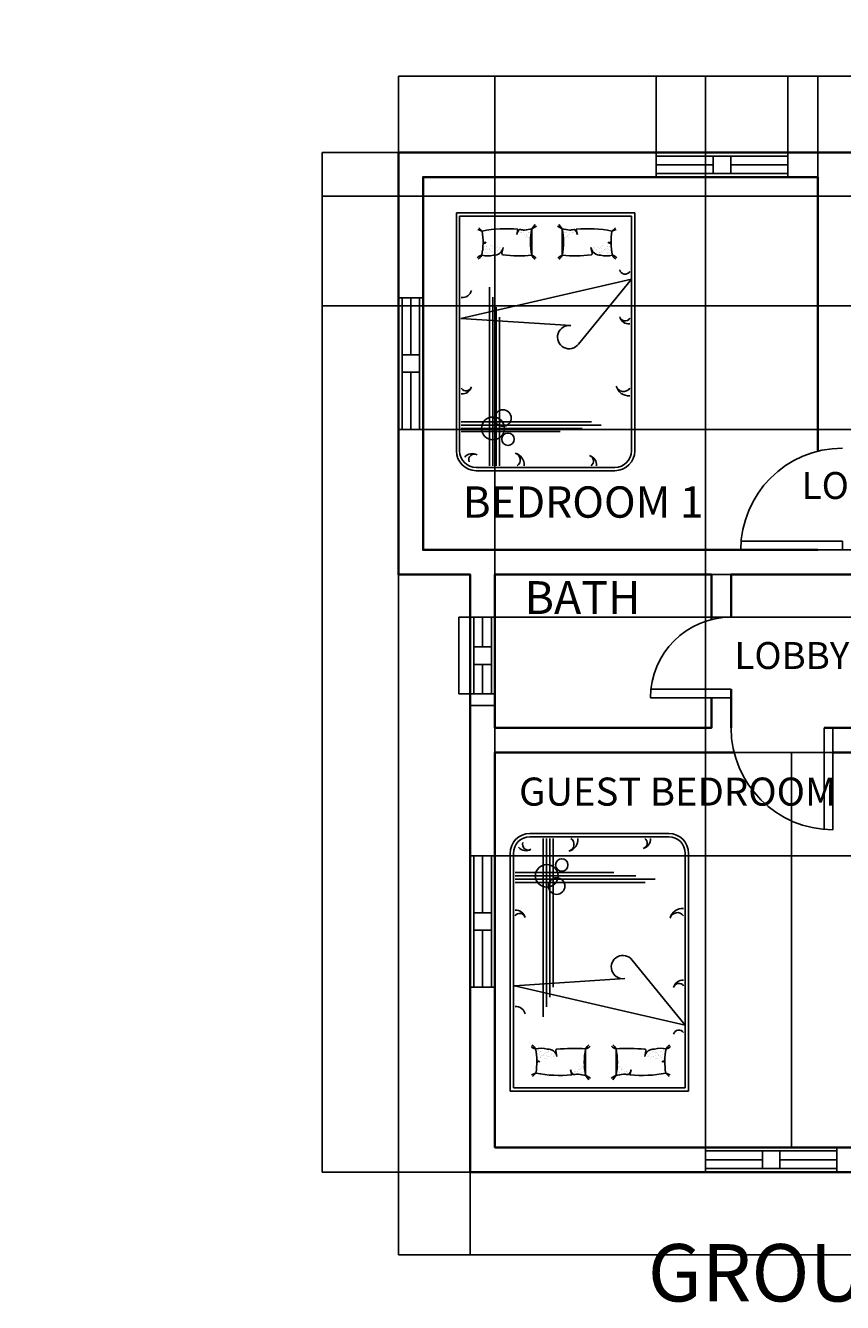
# Model space of a CAD drawing. Units: millimetres. Extents: x 19292 to 100733, y 12374 to 26974.
# Tile 1 of 24: x 19292 to 26744, y 12374 to 24018. Entities that reach past the tile are written whole.
import ezdxf

# ---------------------------------------------------------------- set-up
doc = ezdxf.new("R2010")
doc.units = ezdxf.units.MM
for name, color, linetype, lineweight in [('A-ANNO-DIMS', 2, 'Continuous', 18), ('A-ANNO-TEXT', 7, 'Continuous', 35), ('A-AREA-IDEN', 3, 'Continuous', 25), ('A-DOOR', 4, 'Continuous', 25), ('A-FURN', 8, 'Continuous', 18), ('A-GLAZ', 3, 'Continuous', 25), ('A-WALL', 7, 'Continuous', 35)]:
    doc.layers.add(name, color=color, linetype=linetype, lineweight=lineweight)
doc.layers.add('FURNITURE', color=40, linetype='Continuous')
doc.layers.add('WINDOWS', color=50, linetype='Continuous')
doc.styles.get("Standard").update_dxf_attribs({"font": 'arial.ttf'})
doc.dimstyles.get("Standard").update_dxf_attribs({"dimtxt": 0.18, "dimasz": 0.18, "dimexe": 0.18, "dimexo": 0.0625, "dimgap": 0.09, "dimtad": 0, "dimtih": 1, "dimtoh": 1, "dimdec": 4, "dimzin": 0, "dimdsep": 46, "dimtxsty": 'Standard', "dimcen": 0.09, "dimadec": 0, "dimazin": 0, "dimtfac": 1, "dimtdec": 4, "dimtofl": 0, "dimtmove": 0, "dimatfit": 3, "dimfxl": 1, "dimtolj": 1, "dimtzin": 0, "dimarcsym": 0})

# ---------------------------------------------------------------- blocks, each defined once
blk = doc.blocks.new('WW')
at = {"layer": 'WINDOWS'}
for p, q in [((-5183.867826392408, -4940.876860268414), (-3983.867826392409, -4940.876860268414)), ((-4663.867826392415, -4940.876860268414), (-4663.867826392408, -5100.876860268415)), ((-4503.867826392416, -4940.876860268414), (-4503.867826392408, -5100.876860268415)), ((-4503.867826392416, -4940.876860268414), (-4503.867826392408, -5100.876860268415)), ((-5183.867826392408, -5020.876860268414), (-4663.867826392408, -5020.876860268415)), ((-5183.867826392408, -5100.876860268414), (-3983.867826392409, -5100.876860268414)), ((-4503.867826392416, -5020.876860268414), (-3983.867826392409, -5020.876860268414))]:
    blk.add_line(p, q, dxfattribs=at)
for points in [[(-5183.867826392408, -5133.376860268413), (-5183.867826392408, -4908.376860268414)], [(-3983.867826392409, -4908.376860268414), (-3983.867826392409, -5133.376860268413)]]:
    blk.add_lwpolyline(points, dxfattribs=at)
blk = doc.blocks.new('WW34')
at = {"layer": 'WINDOWS'}
for p, q in [((6711.282750820508, 3446.0021202598), (7411.282750820508, 3446.0021202598)), ((6981.282750820509, 3446.0021202598), (6981.282750820509, 3286.0021202598)), ((7141.282750820508, 3446.0021202598), (7141.282750820508, 3286.0021202598)), ((6711.282750820508, 3366.0021202598), (6981.282750820509, 3366.0021202598)), ((6711.282750820508, 3286.0021202598), (7411.282750820508, 3286.0021202598)), ((7141.282750820508, 3366.0021202598), (7411.282750820508, 3366.0021202598))]:
    blk.add_line(p, q, dxfattribs=at)
for points in [[(6711.282750820508, 3478.5021202598), (6711.282750820508, 3253.5021202598)], [(7411.282750820508, 3253.5021202598), (7411.282750820508, 3478.5021202598)]]:
    blk.add_lwpolyline(points, dxfattribs=at)
blk = doc.blocks.new('DBED-4FT6')
at = {"layer": 'FURNITURE'}
for p, q in [((-27, 0), (-27, -72)), ((-27, 0), (26.99999999999997, 5.68e-14)), ((27, -72.00000000000023), (26.99999999999997, 5.68e-14)), ((-26, -1), (-26, -72)), ((-26, -1), (26.00000000000003, -0.9999999999997726)), ((-4.134652103803261, -4.817063052123046), (-3.144796483066045, -3.500606371767958)), ((5.060678666421324, -4.817063052123046), (4.070823045684107, -3.500606371767958)), ((26, -72.00000000000023), (26.00000000000003, -0.9999999999997726)), ((-19.18306202227052, -5.485972547936796), (-20.50060919072149, -4.967335516912726)), ((-19.18306202227052, -5.485972547936967), (-20.20772305100416, -4.498686779813965)), ((-8.713720467787255, -6.492365964457349), (-8.352181760678093, -4.952469549742318)), ((-8.40590424041818, -6.637378314066779), (-8.40590424041818, -6.637378314066779)), ((-8.239079784370745, -5.562538396824265), (-8.239079784370745, -5.562538396824265)), ((-7.82267294259384, -5.507717396091834), (-7.82267294259384, -5.507717396091834)), ((-7.611546033681406, -5.809807366600068), (-7.611546033681406, -5.809807366600068)), ((-7.515425131198753, -5.088011999378352), (-7.515425131198753, -5.088011999378352)), ((-7.374544898039516, -5.845988456355428), (-7.374544898039516, -5.845988456355428)), ((-7.367969663836447, -5.22313004090148), (-7.367969663836447, -5.22313004090148)), ((-7.274189455356292, -6.024727209938816), (-7.274189455356292, -6.024727209938816)), ((-6.736049374527851, -5.364660689418656), (-6.736049374527851, -5.364660689418656)), ((-6.571710140081449, -5.952767465126385), (-6.571710140081449, -5.952767465126385)), ((-6.245189668756381, -6.559531928114552), (-6.245189668756381, -6.559531928114552)), ((-6.085661545466621, -5.279035507322305), (-6.085661545466621, -5.279035507322305)), ((-5.998452499838663, -7.338874652100457), (-5.998452499838663, -7.338874652100457)), ((-5.875720334132552, -6.590524621115605), (-5.875720334132552, -6.590524621115605)), ((-5.728264866770928, -6.725642662638733), (-5.728264866770928, -6.725642662638733)), ((-5.688613537228434, -7.034850473630854), (-5.688613537228434, -7.034850473630854)), ((-5.669254703689716, -5.224214506589873), (-5.669254703689716, -5.224214506589873)), ((-5.348064670777432, -7.253249470004163), (-5.348064670777432, -7.253249470004163)), ((-5.280472006961815, -5.819278030439932), (-5.280472006961815, -5.819278030439932)), ((-5.230077320474265, -7.360737045650239), (-5.230077320474265, -7.360737045650239)), ((-5.120232544280042, -5.805280123770785), (-5.120232544280042, -5.805280123770785)), ((-4.93200534301593, -7.455280086863638), (-4.93200534301593, -7.455280086863638)), ((-4.931657828999789, -7.198428469271675), (-4.931657828999789, -7.198428469271675)), ((-4.782875965954929, -6.020199967109533), (-4.782875965954929, -6.020199967109533)), ((-4.582631135623728, -5.081157799916695), (-4.582631135623728, -5.081157799916695)), ((-4.249112664583094, -5.02788817272858), (-4.249112664583094, -5.02788817272858)), ((-4.134652103803261, -4.817063052122875), (-2.713769052616612, -3.999588591179417)), ((5.060678666421324, -4.817063052122875), (3.639795615234675, -3.999588591179417)), ((5.175139227201157, -5.027888172729319), (5.175139227201157, -5.027888172729319)), ((5.50865769824179, -5.081157799916638), (5.50865769824179, -5.081157799916638)), ((5.708902528572991, -6.020199967109817), (5.708902528572991, -6.020199967109817)), ((5.857684391617851, -7.198428469271505), (5.857684391617851, -7.198428469271505)), ((5.85803190563331, -7.455280086863353), (5.85803190563331, -7.455280086863353)), ((6.046259106898105, -5.805280123771126), (6.046259106898105, -5.805280123771126)), ((6.156103883091589, -7.360737045650921), (6.156103883091589, -7.360737045650921)), ((6.206498569579878, -5.819278030440671), (6.206498569579878, -5.819278030440671)), ((6.274091233394756, -7.253249470003993), (6.274091233394756, -7.253249470003993)), ((6.595281266307779, -5.224214506589817), (6.595281266307779, -5.224214506589817)), ((6.614640099846496, -7.034850473631365), (6.614640099846496, -7.034850473631365)), ((6.654291429388308, -6.725642662638449), (6.654291429388308, -6.725642662638449)), ((6.801746896750614, -6.590524621115321), (6.801746896750614, -6.590524621115321)), ((6.924479062455986, -7.338874652100287), (6.924479062455986, -7.338874652100287)), ((7.011688108084683, -5.279035507322305), (7.011688108084683, -5.279035507322305)), ((7.171216231373705, -6.559531928115234), (7.171216231373705, -6.559531928115234)), ((7.497736702698773, -5.952767465126157), (7.497736702698773, -5.952767465126157)), ((7.662075937145914, -5.364660689418599), (7.662075937145914, -5.364660689418599)), ((8.200216017975094, -6.024727209939328), (8.200216017975094, -6.024727209939328)), ((8.293996226453771, -5.223130040901196), (8.293996226453771, -5.223130040901196)), ((8.30057146065684, -5.84598845635628), (8.30057146065684, -5.84598845635628)), ((8.441451693816077, -5.088011999378068), (8.441451693816077, -5.088011999378068)), ((8.537572596300208, -5.80980736660058), (8.537572596300208, -5.80980736660058)), ((8.748699505211903, -5.507717396091777), (8.748699505211903, -5.507717396091777)), ((9.165106346988807, -5.562538396824265), (9.165106346988807, -5.562538396824265)), ((9.639747030405317, -6.492365964457349), (9.278208323295416, -4.952469549742318)), ((9.331930803035561, -6.637378314067632), (9.331930803035561, -6.637378314067632)), ((20.10908858488784, -5.485972547936967), (21.13374961362223, -4.498686779813965)), ((20.10908858488858, -5.485972547936796), (21.42663575333882, -4.967335516912726)), ((-18.77590810264172, -9.83900715250769), (-18.77590810264172, -9.83900715250769)), ((-18.7469186025819, -9.831933062623136), (-18.7469186025819, -9.831933062623136)), ((-18.69652391609435, -11.37339207783361), (-18.69652391609435, -11.37339207783361)), ((-18.59621655837128, -9.4634697248635), (-18.59621655837128, -9.4634697248635)), ((-18.43855152431661, -10.05392699584638), (-18.43855152431661, -10.05392699584638)), ((-18.181365058572, -11.01410595179413), (-18.181365058572, -11.01410595179413)), ((-17.90022675242233, -10.10122688085266), (-17.90022675242233, -10.10122688085266)), ((-17.75277128506002, -10.23634492237579), (-17.75277128506002, -10.23634492237579)), ((-17.73180625429978, -10.63313818015905), (-17.73180625429978, -10.63313818015905)), ((-17.53097722951077, -10.92848076969778), (-17.53097722951077, -10.92848076969778)), ((-17.11457038773386, -10.87365976896535), (-17.11457038773386, -10.87365976896535)), ((-16.95651176130502, -10.9659823466007), (-16.95651176130502, -10.9659823466007)), ((-16.85297560618875, -11.06405025953836), (-16.85297560618875, -11.06405025953836)), ((-16.70044691192106, -9.841748322447756), (-16.70044691192106, -9.841748322447756)), ((-16.65005222543351, -11.38320733765818), (-16.65005222543351, -11.38320733765818)), ((-16.2845946132411, -9.834479909678294), (-16.2845946132411, -9.834479909678294)), ((-16.02794681966861, -10.73060306229217), (-16.02794681966861, -10.73060306229217)), ((-15.94723803491598, -10.04939975301698), (-15.94723803491598, -10.04939975301698)), ((-15.57109168263798, -10.55529179420631), (-15.57109168263798, -10.55529179420631)), ((-15.37755899060738, -10.64497788019582), (-15.37755899060738, -10.64497788019582)), ((-14.96115214883048, -10.59015687946339), (-14.96115214883048, -10.59015687946339)), ((-14.55597933435581, -11.35649691174245), (-14.55597933435581, -11.35649691174245)), ((-14.55161047764721, -10.26384189465318), (-14.55161047764721, -10.26384189465318)), ((-14.36166211678738, -11.05952301670902), (-14.36166211678738, -11.05952301670902)), ((-13.87452858076449, -10.44710017279021), (-13.87452858076449, -10.44710017279021)), ((-13.85562067169906, -10.9015990506424), (-13.85562067169906, -10.9015990506424)), ((-13.70816520433675, -11.03671709216553), (-13.70816520433675, -11.03671709216553)), ((-13.52461999197714, -10.56510705403116), (-13.52461999197714, -10.56510705403116)), ((-12.80860301424707, -10.50441610444505), (-13.20654336081225, -12.19935747834682)), ((13.73462957686513, -10.50441610444505), (14.13256992343031, -12.19935747834682)), ((14.45064655459447, -10.56510705403201), (14.45064655459447, -10.56510705403201)), ((14.63419176695407, -11.03671709216536), (14.63419176695407, -11.03671709216536)), ((14.78164723431638, -10.90159905064223), (14.78164723431638, -10.90159905064223)), ((14.80055514338181, -10.44710017278998), (14.80055514338181, -10.44710017278998)), ((15.28768867940545, -11.05952301670942), (15.28768867940545, -11.05952301670942)), ((15.47763704026454, -10.26384189465307), (15.47763704026454, -10.26384189465307)), ((15.48200589697319, -11.35649691174331), (15.48200589697319, -11.35649691174331)), ((15.8871787114478, -10.59015687946316), (15.8871787114478, -10.59015687946316)), ((16.30358555322471, -10.64497788019565), (16.30358555322471, -10.64497788019565)), ((16.49711824525531, -10.55529179420722), (16.49711824525531, -10.55529179420722)), ((16.87326459753331, -10.04939975301738), (16.87326459753331, -10.04939975301738)), ((16.95397338228594, -10.73060306229195), (16.95397338228594, -10.73060306229195)), ((17.21062117585842, -9.834479909678635), (17.21062117585842, -9.834479909678635)), ((17.57607878805157, -11.38320733765908), (17.57607878805157, -11.38320733765908)), ((17.62647347453912, -9.841748322448382), (17.62647347453912, -9.841748322448382)), ((17.77900216880681, -11.06405025953882), (17.77900216880681, -11.06405025953882)), ((17.8825383239224, -10.96598234660052), (17.8825383239224, -10.96598234660052)), ((18.04059695035192, -10.87365976896512), (18.04059695035192, -10.87365976896512)), ((18.45700379212883, -10.92848076969761), (18.45700379212883, -10.92848076969761)), ((18.65783281691711, -10.63313818015967), (18.65783281691711, -10.63313818015967)), ((18.6787978476774, -10.23634492237556), (18.6787978476774, -10.23634492237556)), ((18.82625331503971, -10.10122688085243), (18.82625331503971, -10.10122688085243)), ((19.10739162119006, -11.01410595179391), (19.10739162119006, -11.01410595179391)), ((19.36457808693467, -10.05392699584672), (19.36457808693467, -10.05392699584672)), ((19.5222431209886, -9.463469724863273), (19.5222431209886, -9.463469724863273)), ((19.62255047871167, -11.37339207783429), (19.62255047871167, -11.37339207783429)), ((19.67294516519922, -9.831933062623932), (19.67294516519922, -9.831933062623932)), ((19.70193466525978, -9.839007152508032), (19.70193466525978, -9.839007152508032)), ((-18.66542323901467, -12.3058799545372), (-18.66542323901467, -12.3058799545372)), ((-18.6461292296068, -12.91485109304403), (-18.6461292296068, -12.91485109304403)), ((-18.51796777165236, -12.44099799606033), (-18.51796777165236, -12.44099799606033)), ((-18.12980541361923, -11.84228893838752), (-18.12980541361923, -11.84228893838752)), ((-17.79244883529407, -12.05720878172627), (-17.79244883529407, -12.05720878172627)), ((-17.68141156781223, -12.17459719536947), (-17.68141156781223, -12.17459719536947)), ((-17.44376818388207, -12.98831991447582), (-17.44376818388207, -12.98831991447582)), ((-16.79338035482089, -12.90269473237953), (-16.79338035482089, -12.90269473237953)), ((-16.59965753894596, -12.92466635286894), (-16.59965753894596, -12.92466635286894)), ((-16.37697351304393, -12.84787373164704), (-16.37697351304393, -12.84787373164704)), ((-16.26052195535686, -11.60373950258992), (-16.26052195535686, -11.60373950258992)), ((-16.11306648799456, -11.73885754411304), (-16.11306648799456, -11.73885754411304)), ((-15.63849192421787, -11.83776169555784), (-15.63849192421787, -11.83776169555784)), ((-15.52069699614969, -12.09675080941707), (-15.52069699614969, -12.09675080941707)), ((-15.31680696423956, -12.46849496833795), (-15.31680696423956, -12.46849496833795)), ((-15.3011353458927, -12.05268153889659), (-15.3011353458927, -12.05268153889659)), ((-15.29034994497795, -12.70481702497386), (-15.29034994497795, -12.70481702497386)), ((16.21637650759675, -12.70481702497392), (16.21637650759675, -12.70481702497392)), ((16.22716190851076, -12.05268153889693), (16.22716190851076, -12.05268153889693)), ((16.24283352685688, -12.46849496833772), (16.24283352685688, -12.46849496833772)), ((16.44672355876702, -12.09675080941792), (16.44672355876702, -12.09675080941792)), ((16.56451848683594, -11.83776169555824), (16.56451848683594, -11.83776169555824)), ((17.03909305061188, -11.73885754411276), (17.03909305061188, -11.73885754411276)), ((17.18654851797419, -11.60373950258963), (17.18654851797419, -11.60373950258963)), ((17.303000075662, -12.8478737316471), (17.303000075662, -12.8478737316471)), ((17.52568410156328, -12.92466635286979), (17.52568410156328, -12.92466635286979)), ((17.71940691743896, -12.90269473237953), (17.71940691743896, -12.90269473237953)), ((18.36979474650013, -12.98831991447588), (18.36979474650013, -12.98831991447588)), ((18.60743813042956, -12.17459719537038), (18.60743813042956, -12.17459719537038)), ((18.71847539791213, -12.05720878172661), (18.71847539791213, -12.05720878172661)), ((19.0558319762373, -11.84228893838792), (19.0558319762373, -11.84228893838792)), ((19.44399433426969, -12.4409979960601), (19.44399433426969, -12.4409979960601)), ((19.57215579222412, -12.91485109304494), (19.57215579222412, -12.91485109304494)), ((19.59144980163199, -12.30587995453698), (19.59144980163199, -12.30587995453698)), ((25.99999999999997, -20.04251490499428), (-25.62857142857144, -31.89664668985566)), ((-16.98298633143713, -76.49999999999977), (-16.98298633143804, -22.5)), ((9.968437092424097, -39.68281460107684), (25.99999999999997, -20.04251490499428)), ((-15.98298633143713, -76.49999999999977), (-15.98298633143804, -25.49999999999978)), ((-14.98298633143713, -76.49999999999977), (-14.98298633143804, -28.5)), ((-25.62857142857075, -31.89664668985566), (7.69367787486118, -34.10856123257989)), ((-13.98298633143713, -76.49999999999977), (-13.98298633143804, -31.5)), ((13.92237160184822, -63.18866900046464), (-25.5, -63.18866900046464)), ((16.878192650664, -64.18866900046464), (-25.5, -64.18866900046464)), ((11.10090459947105, -65.18866900046442), (-25.5, -65.18866900046464)), ((4.383130216417612, -66.18866900046442), (-25.5, -66.18866900046464)), ((-21, -77), (21, -77.0000000000002)), ((-21, -78), (21, -78.0000000000002))]:
    blk.add_line(p, q, dxfattribs=at)
for centre, radius in [((-15.90739414396376, -65.18866900046464), 3.437232026160017), ((-12.91182106300494, -62.08454274520204), 2.504372971601696), ((-11.36543750832788, -68.48173730478015), 1.878279728701272)]:
    blk.add_circle(centre, radius, dxfattribs=at)
for centre, radius, start, end in [((-39.10651142374138, -8.817063052122649), 20.20000000000147, 348.6069698988843, 9.491743103753544), ((-11.96490980142209, -41.81687628144138), 37.041008187906, 84.4028612645958, 101.2370836512883), ((-4.825879607851106, -7.608979000930446), 4.045013130436864, 139.9097590679286, 163.9755921234989), ((-11.52336853637479, -33.34663058587759), 28.57069839034993, 80.1409392097565, 82.7553866503384), ((-6.494365647111578, -4.409680956092984), 0.8, 260.1409392097565, 276.031827105606), ((-67.64177770808838, 360.6114736163754), 370.9058781068297, 279.5022474872839, 279.8588573948661), ((15.66534789619453, -8.817063052122135), 20.19999999999818, 168.5788137250011, 191.4211862750058), ((15.66534789619817, -8.817063052122649), 20.20000000000147, 168.5788137249941, 191.4211862750058), ((42751.26187429979, -8.817063056011648), 42755.39671351448, 179.9946396680611, 180.0053603319291), ((-14.73932133358011, -8.817063052122649), 20.20000000000147, 348.5788137249941, 11.42118627500586), ((-42750.33584773717, -8.817063056011648), 42755.39671351448, 359.9946396680676, 0.0053603319421324), ((-14.73932133357721, -8.817063052122135), 20.19999999999818, 348.5788137249941, 11.42118627499883), ((68.56780427070572, 360.6114736163754), 370.9058781068297, 260.141142605134, 260.4977525127162), ((7.420392209728902, -4.409680956092984), 0.8, 263.968172894394, 279.8590607902435), ((12.44939509899285, -33.34663058587759), 28.57069839034993, 97.2446133496616, 99.8590607902435), ((5.751906170469169, -7.608979000930446), 4.045013130436864, 16.0244078765011, 40.09024093207139), ((12.89093636403942, -41.81687628144138), 37.041008187906, 78.76291634871168, 95.59713873540417), ((40.03253798635941, -8.817063052122649), 20.20000000000147, 170.5082568962464, 191.3930301011157), ((-18.63439747950781, -8.362835026573748), 0.7823789253415179, 249.4968528373028, 325.7977956221763), ((-18.4002510232591, -8.445355047199143), 0.5460297530620258, 201.8040695959829, 319.1334346759098), ((-15.61384730787557, -9.916934814375791), 2.86610010521538, 266.7825255240543, 348.1719149754145), ((16.53987387049363, -9.916934814375791), 2.86610010521538, 191.8280850245854, 273.2174744759457), ((19.32627758587716, -8.445355047199143), 0.5460297530620258, 220.8665653240902, 338.1959304040171), ((19.56042404212513, -8.362835026573748), 0.7823789253415179, 214.2022043778237, 290.5031471626973), ((-18.77582684722529, -15.36188282958866), 2.608691937302173, 101.6935339662269, 136.5635486949323), ((-21.64959486574241, -11.66451602127745), 2.608691937302173, 299.1485263283325, 334.0185410570184), ((-17.59820796861624, -5.617120538590143), 7.389908305163763, 256.6498532633935, 284.285581023734), ((-12.81713200699761, -12.29078393797522), 0.4, 166.787330358343, 262.8769841008062), ((-7.849044883706142, 31.23309670203668), 44.20648468370187, 263.4825574665681, 274.8198866450032), ((-1.728460786103994, -11.80933443470422), 2.608691937302173, 202.7242534275457, 237.5942681562781), ((-4.807664589399962, -15.33744552666542), 2.608691937302173, 40.17924578964186, 75.04926051838007), ((5.733691152018025, -15.33744552666542), 2.608691937302173, 104.9507394816199, 139.8207542103581), ((2.654487348722057, -11.80933443470422), 2.608691937302173, 302.4057318437219, 337.2757465724543), ((8.775071446323466, 31.23309670203668), 44.20648468370187, 265.1801133549968, 276.5174425334318), ((13.74315856961567, -12.29078393797522), 0.4, 277.1230158991938, 13.21266964165692), ((18.52423453123356, -5.617120538590143), 7.389908305163763, 255.7144189762659, 283.3501467366066), ((19.70185340984335, -15.36188282958866), 2.608691937302173, 43.43645130506771, 78.3064660337731), ((22.57562142836048, -11.66451602127745), 2.608691937302173, 205.9814589429815, 240.8514736716675), ((24.08149477166717, -16.81385886181465), 1.693091563593251, 194.451540940981, 326.9105817271671), ((-25.2881588087821, -22.70588367900495), 2.933920970030247, 265.8594053605621, 345.9527428336846), ((7.144201548013711, -37.58406550475044), 3.518672218272346, 81.0159135592615, 323.3831798465962), ((24.08149477166717, -30.96393635208892), 1.693091563593251, 194.451540940981, 326.9105817271671), ((25.28815880878119, -30.6743386403075), 2.933920970030691, 194.0472571663257, 274.140594639438), ((-25.28815880878119, -51.86055593582091), 2.933920970030691, 265.8594053605621, 345.9527428336743), ((-24.08149477166717, -52.15015364760233), 1.693091563593251, 213.0894182728328, 345.548459059019), ((23.60865969555653, -51.81050935983859), 2.257455418124377, 194.451540940981, 326.9105817271699), ((25.21754507837523, -51.42437907746352), 3.911894626707589, 194.0472571663257, 274.140594639438), ((-21, -72), 6, 180, 270), ((-21, -72), 5, 180, 270), ((-22.19032021997464, -75.74024097389656), 2.933920970030691, 59.04725716631266, 140.6216534048161), ((-21.541856402534, -74.6822241448225), 1.69309156359317, 59.45154094095176, 200.6983000057678), ((-9.760470192471985, -74.7268684645835), 2.116364454491481, 303.0894182728446, 75.5484590590127), ((-10.12246733219854, -76.23519851097626), 3.667401212538364, 355.8594053605848, 75.95274283367745), ((21, -72.00000000000023), 5, 270, 0), ((21, -72.00000000000023), 6, 270, 0), ((12.54583364175596, -76.28815880878142), 2.933920970030691, 355.8594053605848, 75.95274283367745), ((12.83543135353738, -75.081494771667), 1.693091563593251, 303.0894182728446, 75.5484590590127)]:
    blk.add_arc(centre, radius, start, end, dxfattribs=at)
blk = doc.blocks.new('DOOR-900')
for p, q in [((927.6984484050844, 79.99993679812906), (-0.0003173588884238, 79.99993679812906)), ((927.6984484050844, -6.32018709439e-05), (927.6984484050844, 79.99993679812906)), ((927.6984484050844, -6.32018636679e-05), (927.6984484050844, 79.99993679813633)), ((927.6984484050844, -6.32018709439e-05), (-0.0003173588884238, -6.32018709439e-05))]:
    blk.add_line(p, q)
blk.add_arc((927.6984484050844, -6.32018709439e-05), 927.6987657639736, 90, 180)
blk = doc.blocks.new('DOOR-750')
for p, q in [((655.272448405085, -6.32018709439e-05), (655.272448405085, 735.2719952907646)), ((735.272448405085, -6.32018709439e-05), (735.272448405085, 735.2719952907646)), ((735.272448405085, -6.32018709439e-05), (655.272448405085, -6.32018709439e-05)), ((735.272448405085, -6.32018709439e-05), (655.272448405085, -6.32018709439e-05))]:
    blk.add_line(p, q)
blk.add_arc((735.272448405085, -6.32018709439e-05), 735.2720584926371, 90, 180)
blk = doc.blocks.new('DOOR-SWING-900')
blk.add_line((927.6985029579554, 927.698603252542), (927.6985029579554, -0.0001625114309718))
blk.add_arc((927.6985029579554, 927.698603252542), 927.6987657639734, 180, 270)
blk = doc.blocks.new('*D36')
at = {"layer": 'A-ANNO-DIMS', "color": 0, "lineweight": -2, "transparency": 16777216}
for p, q in [((23348.75214718676, 18622.8606143543), (23243.63464718677, 18622.8606143543)), ((23243.81464718677, 18622.6806143543), (23243.81464718677, 18273.04374532292)), ((23243.81464718677, 17923.0406143543), (23243.81464718677, 18272.67748338568)), ((23348.75214718676, 17922.8606143543), (23243.63464718677, 17922.8606143543))]:
    blk.add_line(p, q, dxfattribs=at)
at = {"layer": 'A-ANNO-DIMS', "color": 0, "transparency": 16777216}
for points in [[(23243.78464718677, 18622.6806143543), (23243.84464718677, 18622.6806143543), (23243.81464718677, 18622.8606143543)], [(23243.78464718677, 17923.0406143543), (23243.84464718677, 17923.0406143543), (23243.81464718677, 17922.8606143543)]]:
    blk.add_solid(points, dxfattribs=at)
at = {"layer": 'Defpoints', "color": 0, "transparency": 16777216}
for p in [(23348.81464718676, 18622.8606143543), (23243.81464718677, 17922.8606143543), (23348.81464718676, 17922.8606143543)]:
    blk.add_point(p, dxfattribs=at)
at = {"layer": 'A-ANNO-DIMS', "color": 0, "transparency": 16777216, "insert": (23243.81464718677, 18272.86061435429), "char_height": 0.18, "attachment_point": 5}
blk.add_mtext('\\A1;WINDOW 700 700 TYP.', dxfattribs=at)
blk = doc.blocks.new('*D37')
at = {"layer": 'A-ANNO-DIMS', "color": 0, "lineweight": -2, "transparency": 16777216}
for p, q in [((23348.81464718675, 17922.79811435429), (23348.81464718675, 17817.68061435429)), ((23348.99464718675, 17817.86061435429), (23460.71509739139, 17817.86061435429)), ((23573.63464718675, 17817.86061435429), (23461.91419698211, 17817.86061435429)), ((23573.81464718675, 17922.79811435429), (23573.81464718675, 17817.68061435429))]:
    blk.add_line(p, q, dxfattribs=at)
at = {"layer": 'A-ANNO-DIMS', "color": 0, "transparency": 16777216}
for points in [[(23348.99464718675, 17817.89061435429), (23348.99464718675, 17817.83061435429), (23348.81464718675, 17817.86061435429)], [(23573.63464718675, 17817.89061435429), (23573.63464718675, 17817.83061435429), (23573.81464718675, 17817.86061435429)]]:
    blk.add_solid(points, dxfattribs=at)
at = {"layer": 'Defpoints', "color": 0, "transparency": 16777216}
for p in [(23348.81464718675, 17922.86061435429), (23573.81464718675, 17922.86061435429), (23573.81464718675, 17817.86061435429)]:
    blk.add_point(p, dxfattribs=at)
at = {"layer": 'A-ANNO-DIMS', "color": 0, "transparency": 16777216, "insert": (23461.31464718675, 17817.86061435429), "char_height": 0.18, "attachment_point": 5}
blk.add_mtext('\\A1;225 TYP.', dxfattribs=at)
blk = doc.blocks.new('*D58')
at = {"layer": 'A-ANNO-DIMS', "color": 0, "lineweight": -2, "transparency": 16777216}
for p, q in [((22694.132448, 22860.787437), (22694.132448, 23555.904937)), ((22694.312448, 23555.724937), (23869.72141841542, 23555.724937)), ((25045.849161, 23555.724937), (23870.44019058459, 23555.724937)), ((25046.029161, 22860.787437), (25046.029161, 23555.904937))]:
    blk.add_line(p, q, dxfattribs=at)
at = {"layer": 'A-ANNO-DIMS', "color": 0, "transparency": 16777216}
for points in [[(22694.312448, 23555.754937), (22694.312448, 23555.694937), (22694.132448, 23555.724937)], [(25045.849161, 23555.754937), (25045.849161, 23555.694937), (25046.029161, 23555.724937)]]:
    blk.add_solid(points, dxfattribs=at)
at = {"layer": 'Defpoints', "color": 0, "transparency": 16777216}
for p in [(25046.029161, 23555.724937), (22694.132448, 22860.724937), (25046.029161, 22860.724937)]:
    blk.add_point(p, dxfattribs=at)
at = {"layer": 'A-ANNO-DIMS', "color": 0, "transparency": 16777216, "insert": (23870.0808045, 23555.724937), "char_height": 0.18, "attachment_point": 5}
blk.add_mtext('\\A1;2352', dxfattribs=at)
blk = doc.blocks.new('*D59')
at = {"layer": 'A-ANNO-DIMS', "color": 0, "lineweight": -2, "transparency": 16777216}
for p, q in [((25046.029161, 22860.787437), (25046.029161, 23555.904937)), ((25046.209161, 23555.724937), (25645.67916782128, 23555.724937)), ((26245.849161, 23555.724937), (25646.37915417872, 23555.724937)), ((26246.029161, 22860.787437), (26246.029161, 23555.904937))]:
    blk.add_line(p, q, dxfattribs=at)
at = {"layer": 'A-ANNO-DIMS', "color": 0, "transparency": 16777216}
for points in [[(25046.209161, 23555.754937), (25046.209161, 23555.694937), (25046.029161, 23555.724937)], [(26245.849161, 23555.754937), (26245.849161, 23555.694937), (26246.029161, 23555.724937)]]:
    blk.add_solid(points, dxfattribs=at)
at = {"layer": 'Defpoints', "color": 0, "transparency": 16777216}
for p in [(26246.029161, 23555.724937), (25046.029161, 22860.724937), (26246.029161, 22860.724937)]:
    blk.add_point(p, dxfattribs=at)
at = {"layer": 'A-ANNO-DIMS', "color": 0, "transparency": 16777216, "insert": (25646.029161, 23555.724937), "char_height": 0.18, "attachment_point": 5}
blk.add_mtext('\\A1;1200', dxfattribs=at)
blk = doc.blocks.new('*D60')
at = {"layer": 'A-ANNO-DIMS', "color": 0, "lineweight": -2, "transparency": 16777216}
for p, q in [((26246.029161, 22860.787437), (26246.029161, 23555.904937)), ((26246.209161, 23555.724937), (26382.20293956139, 23555.724937)), ((26518.952448, 23555.724937), (26382.95866943861, 23555.724937)), ((26519.132448, 22635.787437), (26519.132448, 23555.904937))]:
    blk.add_line(p, q, dxfattribs=at)
at = {"layer": 'A-ANNO-DIMS', "color": 0, "transparency": 16777216}
for points in [[(26246.209161, 23555.754937), (26246.209161, 23555.694937), (26246.029161, 23555.724937)], [(26518.952448, 23555.754937), (26518.952448, 23555.694937), (26519.132448, 23555.724937)]]:
    blk.add_solid(points, dxfattribs=at)
at = {"layer": 'Defpoints', "color": 0, "transparency": 16777216}
for p in [(26519.132448, 23555.724937), (26246.029161, 22860.724937), (26519.132448, 22635.724937)]:
    blk.add_point(p, dxfattribs=at)
at = {"layer": 'A-ANNO-DIMS', "color": 0, "transparency": 16777216, "insert": (26382.5808045, 23555.724937), "char_height": 0.18, "attachment_point": 5}
blk.add_mtext('\\A1;273.1', dxfattribs=at)
blk = doc.blocks.new('*D61')
at = {"layer": 'A-ANNO-DIMS', "color": 0, "lineweight": -2, "transparency": 16777216}
for p, q in [((26519.132448, 22635.787437), (26519.132448, 23555.904937)), ((26519.312448, 23555.724937), (27443.78245482128, 23555.724937)), ((28368.952448, 23555.724937), (27444.48244117872, 23555.724937)), ((28369.132448, 22860.787437), (28369.132448, 23555.904937))]:
    blk.add_line(p, q, dxfattribs=at)
at = {"layer": 'A-ANNO-DIMS', "color": 0, "transparency": 16777216}
for points in [[(26519.312448, 23555.754937), (26519.312448, 23555.694937), (26519.132448, 23555.724937)], [(28368.952448, 23555.754937), (28368.952448, 23555.694937), (28369.132448, 23555.724937)]]:
    blk.add_solid(points, dxfattribs=at)
at = {"layer": 'Defpoints', "color": 0, "transparency": 16777216}
for p in [(28369.132448, 23555.724937), (28369.132448, 22860.724937), (26519.132448, 22635.724937)]:
    blk.add_point(p, dxfattribs=at)
at = {"layer": 'A-ANNO-DIMS', "color": 0, "transparency": 16777216, "insert": (27444.132448, 23555.724937), "char_height": 0.18, "attachment_point": 5}
blk.add_mtext('\\A1;1850', dxfattribs=at)
blk = doc.blocks.new('*D67')
at = {"layer": 'A-ANNO-DIMS', "color": 0, "lineweight": -2, "transparency": 16777216}
for p, q in [((22694.06994800001, 22860.72493700001), (21998.95244800002, 22860.72493700001)), ((21999.13244800002, 22860.54493700001), (21999.13244800002, 18211.91817313779)), ((21999.13244800002, 13562.92760300001), (21999.13244800002, 18211.55436686222)), ((23348.75214700001, 13562.747603), (21998.95244800002, 13562.747603))]:
    blk.add_line(p, q, dxfattribs=at)
at = {"layer": 'A-ANNO-DIMS', "color": 0, "transparency": 16777216}
for points in [[(21999.10244800002, 22860.54493700001), (21999.16244800002, 22860.54493700001), (21999.13244800002, 22860.72493700001)], [(21999.10244800002, 13562.92760300001), (21999.16244800002, 13562.92760300001), (21999.13244800002, 13562.747603)]]:
    blk.add_solid(points, dxfattribs=at)
at = {"layer": 'Defpoints', "color": 0, "transparency": 16777216}
for p in [(22694.13244800001, 22860.72493700001), (21999.13244800002, 13562.747603), (23348.81464700001, 13562.747603)]:
    blk.add_point(p, dxfattribs=at)
at = {"layer": 'A-ANNO-DIMS', "color": 0, "transparency": 16777216, "insert": (21999.13244800002, 18211.73627), "char_height": 0.18, "attachment_point": 5}
blk.add_mtext('\\A1;9298', dxfattribs=at)
blk = doc.blocks.new('*D68')
at = {"layer": 'A-ANNO-DIMS', "color": 0, "lineweight": -2, "transparency": 16777216}
for p, q in [((22919.19494800001, 20335.72493700001), (36879.34896500003, 20335.72493700001)), ((36879.16896500003, 20335.54493700001), (36879.16896500003, 19785.9068401378)), ((36879.16896500003, 19235.90493700001), (36879.16896500003, 19785.54303386222)), ((22919.19494800001, 19235.724937), (36879.34896500003, 19235.72493700001))]:
    blk.add_line(p, q, dxfattribs=at)
at = {"layer": 'A-ANNO-DIMS', "color": 0, "transparency": 16777216}
for points in [[(36879.13896500003, 20335.54493700001), (36879.19896500003, 20335.54493700001), (36879.16896500003, 20335.72493700001)], [(36879.13896500003, 19235.90493700001), (36879.19896500003, 19235.90493700001), (36879.16896500003, 19235.72493700001)]]:
    blk.add_solid(points, dxfattribs=at)
at = {"layer": 'Defpoints', "color": 0, "transparency": 16777216}
for p in [(22919.13244800001, 20335.72493700001), (22919.13244800001, 19235.724937), (36879.16896500003, 19235.72493700001)]:
    blk.add_point(p, dxfattribs=at)
at = {"layer": 'A-ANNO-DIMS', "color": 0, "transparency": 16777216, "insert": (36879.16896500003, 19785.72493699999), "char_height": 0.18, "attachment_point": 5}
blk.add_mtext('\\A1;1100', dxfattribs=at)
blk = doc.blocks.new('*D69')
at = {"layer": 'A-ANNO-DIMS', "color": 0, "lineweight": -2, "transparency": 16777216}
for p, q in [((23573.87714700001, 19012.74760300001), (36879.34896500003, 19012.74760300001)), ((36879.16896500003, 19012.56760300001), (36879.16896500003, 18817.98607302934)), ((36879.16896500003, 18623.04061400001), (36879.16896500003, 18817.62214397068)), ((23573.87714700001, 18622.86061400001), (36879.34896500003, 18622.86061400001))]:
    blk.add_line(p, q, dxfattribs=at)
at = {"layer": 'A-ANNO-DIMS', "color": 0, "transparency": 16777216}
for points in [[(36879.13896500003, 19012.56760300001), (36879.19896500003, 19012.56760300001), (36879.16896500003, 19012.74760300001)], [(36879.13896500003, 18623.04061400001), (36879.19896500003, 18623.04061400001), (36879.16896500003, 18622.86061400001)]]:
    blk.add_solid(points, dxfattribs=at)
at = {"layer": 'Defpoints', "color": 0, "transparency": 16777216}
for p in [(23573.81464700001, 19012.74760300001), (23573.81464700001, 18622.86061400001), (36879.16896500003, 18622.86061400001)]:
    blk.add_point(p, dxfattribs=at)
at = {"layer": 'A-ANNO-DIMS', "color": 0, "transparency": 16777216, "insert": (36879.16896500003, 18817.8041085), "char_height": 0.18, "attachment_point": 5}
blk.add_mtext('\\A1;389.9', dxfattribs=at)
blk = doc.blocks.new('*D70')
at = {"layer": 'A-ANNO-DIMS', "color": 0, "lineweight": -2, "transparency": 16777216}
for p, q in [((23573.87714700001, 17387.747603), (36879.34896500003, 17387.74760300001)), ((36879.16896500003, 17387.56760300001), (36879.16896500003, 16917.9295061378)), ((36879.16896500003, 16447.92760300001), (36879.16896500003, 16917.56569986222)), ((23573.87714700001, 16447.747603), (36879.34896500003, 16447.74760300001))]:
    blk.add_line(p, q, dxfattribs=at)
at = {"layer": 'A-ANNO-DIMS', "color": 0, "transparency": 16777216}
for points in [[(36879.13896500003, 17387.56760300001), (36879.19896500003, 17387.56760300001), (36879.16896500003, 17387.74760300001)], [(36879.13896500003, 16447.92760300001), (36879.19896500003, 16447.92760300001), (36879.16896500003, 16447.74760300001)]]:
    blk.add_solid(points, dxfattribs=at)
at = {"layer": 'Defpoints', "color": 0, "transparency": 16777216}
for p in [(23573.81464700001, 17387.747603), (36879.16896500003, 17387.74760300001), (23573.81464700001, 16447.747603)]:
    blk.add_point(p, dxfattribs=at)
at = {"layer": 'A-ANNO-DIMS', "color": 0, "transparency": 16777216, "insert": (36879.16896500003, 16917.74760299999), "char_height": 0.18, "attachment_point": 5}
blk.add_mtext('\\A1;940', dxfattribs=at)
blk = doc.blocks.new('*D71')
at = {"layer": 'A-ANNO-DIMS', "color": 0, "lineweight": -2, "transparency": 16777216}
for p, q in [((26973.75214700001, 17387.747603), (26278.63464700003, 17387.747603)), ((26278.81464700003, 17387.567603), (26278.81464700003, 15587.92956752933)), ((26278.81464700003, 13787.927603), (26278.81464700003, 15587.56563847067)), ((26973.75214700001, 13787.747603), (26278.63464700003, 13787.747603))]:
    blk.add_line(p, q, dxfattribs=at)
at = {"layer": 'A-ANNO-DIMS', "color": 0, "transparency": 16777216}
for points in [[(26278.78464700003, 17387.567603), (26278.84464700003, 17387.567603), (26278.81464700003, 17387.747603)], [(26278.78464700003, 13787.927603), (26278.84464700003, 13787.927603), (26278.81464700003, 13787.747603)]]:
    blk.add_solid(points, dxfattribs=at)
at = {"layer": 'Defpoints', "color": 0, "transparency": 16777216}
for p in [(26278.81464700003, 17387.747603), (26973.81464700002, 17387.747603), (26973.81464700002, 13787.747603)]:
    blk.add_point(p, dxfattribs=at)
at = {"layer": 'A-ANNO-DIMS', "color": 0, "transparency": 16777216, "insert": (26278.81464700002, 15587.74760299999), "char_height": 0.18, "attachment_point": 5}
blk.add_mtext('\\A1;3600', dxfattribs=at)
blk = doc.blocks.new('*D79')
at = {"layer": 'A-ANNO-DIMS', "color": 0, "lineweight": -2, "transparency": 16777216}
for p, q in [((22694.132448, 22860.662437), (22694.132448, 12808.8126)), ((36144.168965, 15985.662437), (36144.168965, 12808.8126)), ((22694.312448, 12808.9926), (29418.73078835539, 12808.9926)), ((36143.988965, 12808.9926), (29419.57062464461, 12808.9926))]:
    blk.add_line(p, q, dxfattribs=at)
at = {"layer": 'A-ANNO-DIMS', "color": 0, "transparency": 16777216}
for points in [[(22694.312448, 12809.0226), (22694.312448, 12808.9626), (22694.132448, 12808.9926)], [(36143.988965, 12809.0226), (36143.988965, 12808.9626), (36144.168965, 12808.9926)]]:
    blk.add_solid(points, dxfattribs=at)
at = {"layer": 'Defpoints', "color": 0, "transparency": 16777216}
for p in [(22694.132448, 22860.724937), (36144.168965, 15985.724937), (36144.168965, 12808.9926)]:
    blk.add_point(p, dxfattribs=at)
at = {"layer": 'A-ANNO-DIMS', "color": 0, "transparency": 16777216, "insert": (29419.1507065, 12808.9926), "char_height": 0.18, "attachment_point": 5}
blk.add_mtext('\\A1;13450', dxfattribs=at)
blk = doc.blocks.new('*D80')
at = {"layer": 'A-ANNO-DIMS', "color": 0, "lineweight": -2, "transparency": 16777216}
for p, q in [((22694.132448, 19010.662437), (22694.132448, 12808.8126)), ((23348.814647, 19010.662437), (23348.814647, 12808.8126)), ((22694.312448, 12808.9926), (23021.07935241132, 12808.9926)), ((23348.634647, 12808.9926), (23021.86774258867, 12808.9926))]:
    blk.add_line(p, q, dxfattribs=at)
at = {"layer": 'A-ANNO-DIMS', "color": 0, "transparency": 16777216}
for points in [[(22694.312448, 12809.0226), (22694.312448, 12808.9626), (22694.132448, 12808.9926)], [(23348.634647, 12809.0226), (23348.634647, 12808.9626), (23348.814647, 12808.9926)]]:
    blk.add_solid(points, dxfattribs=at)
at = {"layer": 'Defpoints', "color": 0, "transparency": 16777216}
for p in [(22694.132448, 19010.724937), (23348.814647, 19010.724937), (23348.814647, 12808.9926)]:
    blk.add_point(p, dxfattribs=at)
at = {"layer": 'A-ANNO-DIMS', "color": 0, "transparency": 16777216, "insert": (23021.4735475, 12808.9926), "char_height": 0.18, "attachment_point": 5}
blk.add_mtext('\\A1;654.7', dxfattribs=at)
blk = doc.blocks.new('*D81')
at = {"layer": 'A-ANNO-DIMS', "color": 0, "lineweight": -2, "transparency": 16777216}
for p, q in [((23573.814647, 13787.810103), (23573.814647, 23555.904937)), ((23573.994647, 23555.724937), (24533.11907830355, 23555.724937)), ((25493.155174, 23555.724937), (24534.03074269645, 23555.724937)), ((25493.335174, 13787.810103), (25493.335174, 23555.904937))]:
    blk.add_line(p, q, dxfattribs=at)
at = {"layer": 'A-ANNO-DIMS', "color": 0, "transparency": 16777216}
for points in [[(23573.994647, 23555.754937), (23573.994647, 23555.694937), (23573.814647, 23555.724937)], [(25493.155174, 23555.754937), (25493.155174, 23555.694937), (25493.335174, 23555.724937)]]:
    blk.add_solid(points, dxfattribs=at)
at = {"layer": 'Defpoints', "color": 0, "transparency": 16777216}
for p in [(25493.335174, 23555.724937), (23573.814647, 13787.747603), (25493.335174, 13787.747603)]:
    blk.add_point(p, dxfattribs=at)
at = {"layer": 'A-ANNO-DIMS', "color": 0, "transparency": 16777216, "insert": (24533.5749105, 23555.724937), "char_height": 0.18, "attachment_point": 5}
blk.add_mtext('\\A1;1919.5', dxfattribs=at)
blk = doc.blocks.new('*D85')
at = {"layer": 'A-ANNO-DIMS', "color": 0, "lineweight": -2, "transparency": 16777216}
for p, q in [((31169.06994800002, 22460.72493700001), (21998.95244800002, 22460.724937)), ((21999.13244800002, 22460.544937), (21999.13244800002, 21960.90684013779)), ((21999.13244800002, 21460.904937), (21999.13244800002, 21960.54303386222)), ((31169.06994800002, 21460.72493700001), (21998.95244800002, 21460.724937))]:
    blk.add_line(p, q, dxfattribs=at)
at = {"layer": 'A-ANNO-DIMS', "color": 0, "transparency": 16777216}
for points in [[(21999.10244800002, 22460.544937), (21999.16244800002, 22460.544937), (21999.13244800002, 22460.724937)], [(21999.10244800002, 21460.904937), (21999.16244800002, 21460.904937), (21999.13244800002, 21460.724937)]]:
    blk.add_solid(points, dxfattribs=at)
at = {"layer": 'Defpoints', "color": 0, "transparency": 16777216}
for p in [(31169.13244800001, 22460.72493700001), (21999.13244800002, 21460.724937), (31169.13244800001, 21460.72493700001)]:
    blk.add_point(p, dxfattribs=at)
at = {"layer": 'A-ANNO-DIMS', "color": 0, "transparency": 16777216, "insert": (21999.13244800002, 21960.724937), "char_height": 0.18, "attachment_point": 5}
blk.add_mtext('\\A1;1000', dxfattribs=at)

msp = doc.modelspace()

# ---------------------------------------------------------------- linework, layer by layer
at = {"layer": 'A-DOOR'}
msp.add_line((26576.14450295795, 17612.74760325254), (26576.14450295795, 16685.04883748857), dxfattribs=at)
at = {"layer": 'A-WALL'}
for points in [[(29548.57101814721, 14906.40305703235), (27198.81464718675, 14906.40305703235), (27198.81464718675, 13562.74760325254), (23348.81464718675, 13562.74760325254), (23348.81464718675, 19010.72493679813), (22694.13244840509, 19010.72493679813), (22694.13244840509, 22860.72493679813), (28369.13244840509, 22860.72493679813), (28369.13244840509, 21460.72493679813), (31169.13244840509, 21460.72493679812), (31169.13244840509, 22460.72493679813), (34419.13244840509, 22460.72493679813), (34419.13244840509, 22208.02617103415)], [(26519.13244840509, 19235.72493679813), (22919.13244840509, 19235.72493679813), (22919.13244840509, 22635.72493679813), (26519.13244840509, 22635.72493679813), (26519.13244840509, 20135.72493679813)], [(25548.81464718675, 18600.18175280314), (25548.81464718675, 19012.74760325254), (23573.81464718675, 19012.74760325254), (23573.81464718675, 17612.74760325254), (25548.81464718675, 17612.74760325254), (25548.81464718675, 17887.18969709508)], [(26973.81464718675, 18812.74760325254), (26973.81464718675, 19012.74760325254), (25728.44573719398, 19012.74760325254), (25728.44573719398, 18622.46175558771)], [(25728.44573719398, 17967.18969709508), (25728.44573719398, 17612.74760325254)], [(26576.14450295795, 17612.74760325254), (26973.81464718675, 17612.74760325254), (26973.81464718675, 17812.74760325254)], [(25756.14450295796, 17387.74760325254), (23573.81464718675, 17387.74760325254), (23573.81464718675, 13787.74760325254), (26973.81464718675, 13787.74760325254), (26973.81464718675, 17387.74760325254), (26656.14450295795, 17387.74760325254)]]:
    msp.add_lwpolyline(points, dxfattribs=at)

# ---------------------------------------------------------------- block references
at = {"layer": 'A-DOOR'}
for name, p in [('DOOR-900', (25816.434, 19235.725)), ('DOOR-SWING-900', (25728.446, 16685.049))]:
    msp.add_blockref(name, p, dxfattribs=at)
at = {"layer": 'A-DOOR', "extrusion": (0, 0, -1), "zscale": -1, "rotation": 270.0000000000006}
msp.add_blockref('DOOR-750', (-25728.44567399211, 18622.46214550017), dxfattribs=at)
at = {"layer": 'A-FURN', "xscale": 30.13269765108242, "yscale": 30.13269765108242, "zscale": 30.13269765108242}
msp.add_blockref('DBED-4FT6', (24035.78356620017, 22309.03809122464), dxfattribs=at)
at = {"layer": 'A-FURN', "xscale": -30.13269765108242, "yscale": 30.13269765108242, "zscale": 30.13269765108242, "rotation": 180}
msp.add_blockref('DBED-4FT6', (24526.13317827764, 14299.82510942071), dxfattribs=at)
at = {"layer": 'A-GLAZ'}
for p in [(30229.89698776789, 27769.10179706654), (30677.20300003723, 18696.12446352095)]:
    msp.add_blockref('WW', p, dxfattribs=at)
at = {"layer": 'A-GLAZ', "rotation": 270}
for name, p in [('WW', (27827.5093086735, 16351.85711040572)), ('WW34', (20095.31252692695, 25334.1433651748)), ('WW', (28482.19150745516, 11263.87977686013))]:
    msp.add_blockref(name, p, dxfattribs=at)

# ---------------------------------------------------------------- texts
at = {"layer": 'A-ANNO-TEXT'}
msp.add_text('GROUND FLOOR PLAN', height=523.2684807306957, dxfattribs=at).set_placement((24968.61935149389, 12383.03142158251))
at = {"layer": 'A-ANNO-TEXT', "insert": (19292.05708275246, 24018.05555617658), "char_height": 2.5, "attachment_point": 1}
msp.add_mtext_dynamic_manual_height_columns('BEDROOM 1', width=1021.46168757882, gutter_width=12.5, heights=[0], dxfattribs=at)
at = {"layer": 'A-AREA-IDEN'}
for s, height, p in [('LOBBY', 245.4119814836725, (26372.6017782843, 19701.03758517349)), ('BEDROOM 1', 285.4899223852939, (23279.19546794805, 19530.07367181583)), ('BATH', 299.1707480039913, (23844.80913814716, 18652.15274189098)), ('LOBBY', 245.4119814836725, (25758.8009767047, 18150.5208007784)), ('GUEST BEDROOM', 255.9224915282845, (23794.14550739036, 16904.31845452375))]:
    msp.add_text(s, height=height, dxfattribs=at).set_placement(p)

# ---------------------------------------------------------------- dimensions: what is measured, and where the dimension line sits
at = {"layer": 'A-ANNO-DIMS'}
for base, p1, p2, override, picture, middle in [((25046.029161, 23555.724937), (22694.132448, 22860.724937), (25046.029161, 22860.724937), {"dimdec": 0, "dimlfac": 1, "dimrnd": 0, "dimzin": 0, "dimdsep": 46, "dimlunit": 2}, '*D58', (23870.0808045, 23555.724937)), ((25493.335174, 23555.724937), (23573.814647, 13787.747603), (25493.335174, 13787.747603), {"dimdec": 1, "dimlfac": 1, "dimrnd": 0, "dimzin": 0, "dimdsep": 46, "dimlunit": 2}, '*D81', (24533.5749105, 23555.724937)), ((26246.029161, 23555.724937), (25046.029161, 22860.724937), (26246.029161, 22860.724937), {"dimdec": 0, "dimlfac": 1, "dimrnd": 0, "dimzin": 0, "dimdsep": 46, "dimlunit": 2}, '*D59', (25646.029161, 23555.724937)), ((26519.132448, 23555.724937), (26246.029161, 22860.724937), (26519.132448, 22635.724937), {"dimdec": 1, "dimlfac": 1, "dimrnd": 0, "dimzin": 0, "dimdsep": 46, "dimlunit": 2}, '*D60', (26382.5808045, 23555.724937)), ((28369.132448, 23555.724937), (26519.132448, 22635.724937), (28369.132448, 22860.724937), {"dimdec": 0, "dimlfac": 1, "dimrnd": 0, "dimzin": 0, "dimdsep": 46, "dimlunit": 2}, '*D61', (27444.132448, 23555.724937)), ((36144.168965, 12808.9926), (22694.132448, 22860.724937), (36144.168965, 15985.724937), {"dimdec": 0, "dimlfac": 1, "dimrnd": 0, "dimzin": 0, "dimdsep": 46, "dimlunit": 2}, '*D79', (29419.1507065, 12808.9926)), ((23348.814647, 12808.9926), (22694.132448, 19010.724937), (23348.814647, 19010.724937), {"dimdec": 1, "dimlfac": 1, "dimrnd": 0, "dimzin": 0, "dimdsep": 46, "dimlunit": 2}, '*D80', (23021.4735475, 12808.9926))]:
    dim = msp.add_linear_dim(base=base, p1=p1, p2=p2, dimstyle='Standard', override=override, dxfattribs=at)
    dim.commit()
    dim.dimension.update_dxf_attribs({"geometry": picture, "text_midpoint": middle})
for base, p1, p2, override, picture, middle in [((21999.13244800002, 13562.747603), (22694.132448, 22860.724937), (23348.814647, 13562.747603), {"dimdec": 0, "dimlfac": 1, "dimrnd": 0, "dimzin": 0, "dimdsep": 46, "dimlunit": 2}, '*D67', (21999.13244800002, 18211.73627)), ((21999.13244800002, 21460.724937), (31169.132448, 22460.724937), (31169.132448, 21460.724937), {"dimdec": 0, "dimlfac": 1, "dimrnd": 0, "dimzin": 0, "dimdsep": 46, "dimlunit": 2}, '*D85', (21999.13244800002, 21960.724937)), ((36879.16896500003, 19235.72493700001), (22919.132448, 20335.724937), (22919.132448, 19235.724937), {"dimdec": 0, "dimlfac": 1, "dimrnd": 0, "dimzin": 0, "dimdsep": 46, "dimlunit": 2}, '*D68', (36879.16896500003, 19785.72493699999)), ((36879.16896500003, 18622.86061400001), (23573.814647, 19012.747603), (23573.814647, 18622.860614), {"dimdec": 1, "dimlfac": 1, "dimrnd": 0, "dimzin": 0, "dimdsep": 46, "dimlunit": 2}, '*D69', (36879.16896500003, 18817.8041085)), ((36879.16896500003, 17387.74760300001), (23573.814647, 16447.747603), (23573.814647, 17387.747603), {"dimdec": 0, "dimlfac": 1, "dimrnd": 0, "dimzin": 0, "dimdsep": 46, "dimlunit": 2}, '*D70', (36879.16896500003, 16917.74760299999)), ((26278.81464700003, 17387.747603), (26973.814647, 13787.747603), (26973.814647, 17387.747603), {"dimdec": 0, "dimlfac": 1, "dimrnd": 0, "dimzin": 0, "dimdsep": 46, "dimlunit": 2}, '*D71', (26278.81464700002, 15587.74760299999))]:
    dim = msp.add_linear_dim(base=base, p1=p1, p2=p2, angle=90, dimstyle='Standard', override=override, dxfattribs=at)
    dim.commit()
    dim.dimension.update_dxf_attribs({"geometry": picture, "text_midpoint": middle})
dim = msp.add_linear_dim(base=(23243.81464718677, 17922.8606143543), p1=(23348.81464718675, 18622.86061435429), p2=(23348.81464718675, 17922.86061435429), angle=270, text='WINDOW 700 <> TYP.', dimstyle='Standard', override={"dimdec": 0, "dimrnd": 0, "dimzin": 0, "dimlunit": 2}, dxfattribs=at)
dim.commit()
dim.dimension.update_dxf_attribs({"geometry": '*D36', "text_midpoint": (23243.81464718677, 18272.86061435429)})
dim = msp.add_linear_dim(base=(23573.81464718675, 17817.86061435429), p1=(23348.81464718675, 17922.86061435429), p2=(23573.81464718675, 17922.86061435429), text='<> TYP.', dimstyle='Standard', override={"dimdec": 0, "dimrnd": 0, "dimzin": 0, "dimlunit": 2}, dxfattribs=at)
dim.commit()
dim.dimension.update_dxf_attribs({"geometry": '*D37', "text_midpoint": (23461.31464718675, 17817.86061435429)})

doc.saveas('drawing.dxf')
